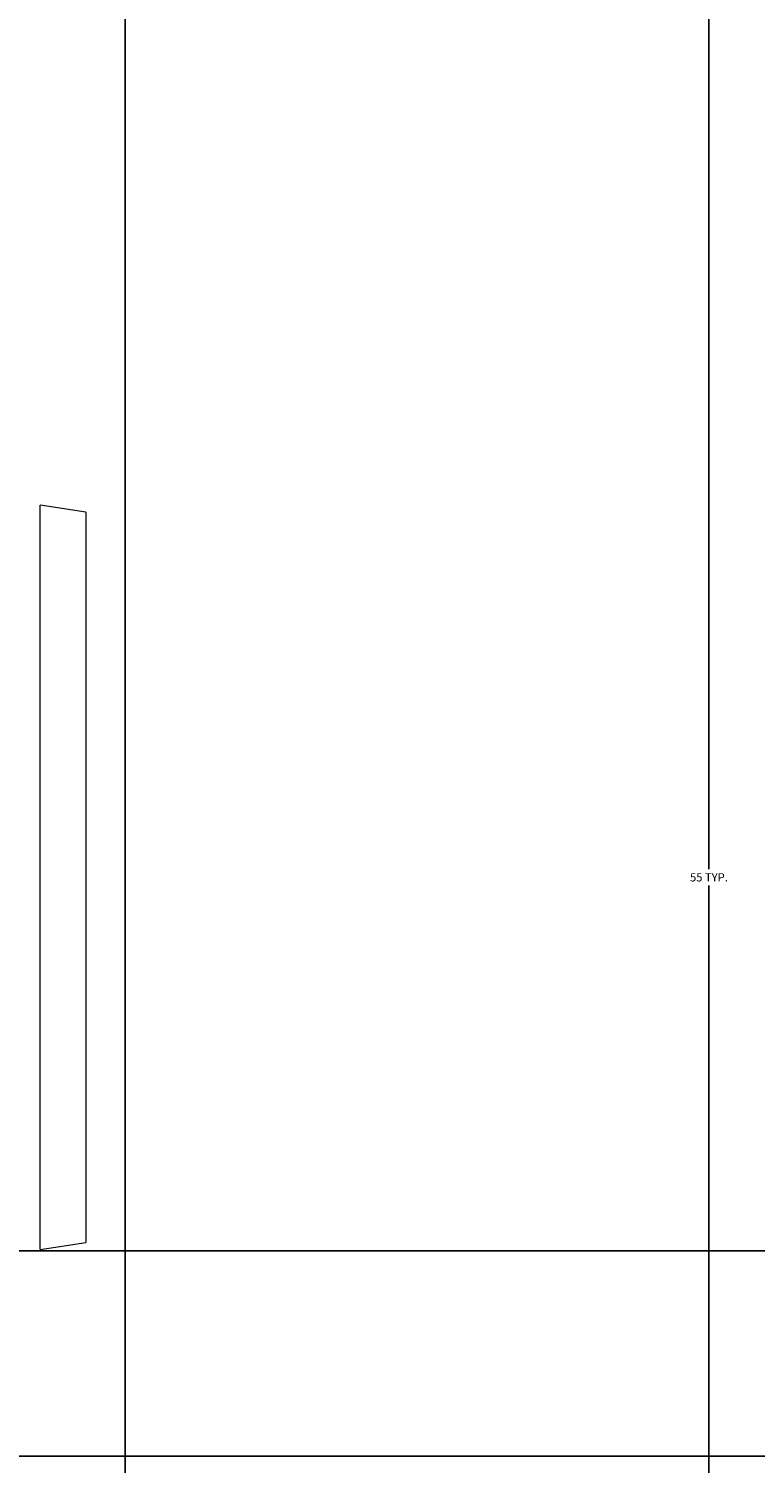
# Model space of a CAD drawing. Units: inches. Extents: x 7359 to 7979, y 33027 to 34263.
# Tile 12 of 32: x 7748 to 7764, y 33386 to 33417. Entities that reach past the tile are written whole.
import ezdxf

# ---------------------------------------------------------------- set-up
doc = ezdxf.new("R2010")
doc.units = ezdxf.units.IN
doc.layers.add('A-ANNO-DIMS', color=2, linetype='Continuous', lineweight=18)
doc.layers.add('A-FURN', color=8, linetype='Continuous', lineweight=18)
doc.styles.get("Standard").update_dxf_attribs({"font": 'arial.ttf'})
doc.dimstyles.get("Standard").update_dxf_attribs({"dimtxt": 0.18, "dimasz": 0.18, "dimexe": 0.18, "dimexo": 0.0625, "dimgap": 0.09, "dimtad": 0, "dimtih": 1, "dimtoh": 1, "dimdec": 4, "dimzin": 0, "dimdsep": 46, "dimtxsty": 'Standard', "dimcen": 0.09, "dimadec": 0, "dimazin": 0, "dimtfac": 1, "dimtdec": 4, "dimtofl": 0, "dimtmove": 0, "dimatfit": 3, "dimfxl": 1, "dimtolj": 1, "dimtzin": 0, "dimarcsym": 0})

# ---------------------------------------------------------------- blocks, each defined once
blk = doc.blocks.new('Dining Set - 36 x 72 in.')
for p, q in [((44.5, -8.15843), (44.5, 8.15338)), ((45.5, 8), (44.5005, 8.15617)), ((45.5, 8), (45.5, -8)), ((44.4997, -8.15631), (45.5, -8))]:
    blk.add_line(p, q)
blk = doc.blocks.new('*D37')
at = {"layer": 'A-ANNO-DIMS', "color": 0, "lineweight": -2, "transparency": 16777216}
for p, q in [((7748.925, 33426.344), (7762.693, 33426.344)), ((7762.513, 33426.164), (7762.513, 33399.025)), ((7762.513, 33371.524), (7762.513, 33398.662)), ((7748.925, 33371.344), (7762.693, 33371.344))]:
    blk.add_line(p, q, dxfattribs=at)
at = {"layer": 'A-ANNO-DIMS', "color": 0, "transparency": 16777216}
for points in [[(7762.483, 33426.164), (7762.543, 33426.164), (7762.513, 33426.344)], [(7762.483, 33371.524), (7762.543, 33371.524), (7762.513, 33371.344)]]:
    blk.add_solid(points, dxfattribs=at)
at = {"layer": 'Defpoints', "color": 0, "transparency": 16777216}
for p in [(7748.863, 33426.344), (7762.513, 33426.344), (7748.863, 33371.344)]:
    blk.add_point(p, dxfattribs=at)
at = {"layer": 'A-ANNO-DIMS', "color": 0, "transparency": 16777216, "insert": (7762.513, 33398.844), "char_height": 0.18, "attachment_point": 5}
blk.add_mtext('\\A1;55 TYP.', dxfattribs=at)
blk = doc.blocks.new('*D74')
at = {"layer": 'A-ANNO-DIMS', "color": 0, "lineweight": -2, "transparency": 16777216}
for p, q in [((7743.727, 33618.1), (7743.727, 33027.177)), ((7787.034, 33618.1), (7787.034, 33027.177)), ((7743.907, 33027.357), (7765, 33027.357)), ((7786.854, 33027.357), (7765.76, 33027.357))]:
    blk.add_line(p, q, dxfattribs=at)
at = {"layer": 'A-ANNO-DIMS', "color": 0, "transparency": 16777216}
for points in [[(7743.907, 33027.387), (7743.907, 33027.327), (7743.727, 33027.357)], [(7786.854, 33027.387), (7786.854, 33027.327), (7787.034, 33027.357)]]:
    blk.add_solid(points, dxfattribs=at)
at = {"layer": 'Defpoints', "color": 0, "transparency": 16777216}
for p in [(7743.727, 33618.162), (7787.034, 33618.162), (7787.034, 33027.357)]:
    blk.add_point(p, dxfattribs=at)
at = {"layer": 'A-ANNO-DIMS', "color": 0, "transparency": 16777216, "insert": (7765.38, 33027.357), "char_height": 0.18, "attachment_point": 5}
blk.add_mtext('\\A1;43.31', dxfattribs=at)
blk = doc.blocks.new('*D85')
at = {"layer": 'A-ANNO-DIMS', "color": 0, "lineweight": -2, "transparency": 16777216}
for p, q in [((7793.064, 33390.662), (7369.542, 33390.662)), ((7369.722, 33390.482), (7369.722, 33388.594)), ((7369.722, 33386.342), (7369.722, 33388.231)), ((7793.064, 33386.162), (7369.542, 33386.162))]:
    blk.add_line(p, q, dxfattribs=at)
at = {"layer": 'A-ANNO-DIMS', "color": 0, "transparency": 16777216}
for points in [[(7369.692, 33390.482), (7369.752, 33390.482), (7369.722, 33390.662)], [(7369.692, 33386.342), (7369.752, 33386.342), (7369.722, 33386.162)]]:
    blk.add_solid(points, dxfattribs=at)
at = {"layer": 'Defpoints', "color": 0, "transparency": 16777216}
for p in [(7793.127, 33390.662), (7369.722, 33386.162), (7793.127, 33386.162)]:
    blk.add_point(p, dxfattribs=at)
at = {"layer": 'A-ANNO-DIMS', "color": 0, "transparency": 16777216, "insert": (7369.722, 33388.412), "char_height": 0.18, "attachment_point": 5}
blk.add_mtext('\\A1;4.5', dxfattribs=at)
blk = doc.blocks.new('*D87')
at = {"layer": 'A-ANNO-DIMS', "color": 0, "lineweight": -2, "transparency": 16777216}
for p, q in [((7743.726578, 33453.099789), (7743.726578, 33027.176807)), ((7749.726578, 33453.099789), (7749.726578, 33027.176807)), ((7743.906578, 33027.356807), (7746.577151, 33027.356807)), ((7749.546578, 33027.356807), (7746.876005, 33027.356807))]:
    blk.add_line(p, q, dxfattribs=at)
at = {"layer": 'A-ANNO-DIMS', "color": 0, "transparency": 16777216}
for points in [[(7743.906578, 33027.386807), (7743.906578, 33027.326807), (7743.726578, 33027.356807)], [(7749.546578, 33027.386807), (7749.546578, 33027.326807), (7749.726578, 33027.356807)]]:
    blk.add_solid(points, dxfattribs=at)
at = {"layer": 'Defpoints', "color": 0, "transparency": 16777216}
for p in [(7743.726578, 33453.162289), (7749.726578, 33453.162289), (7749.726578, 33027.356807)]:
    blk.add_point(p, dxfattribs=at)
at = {"layer": 'A-ANNO-DIMS', "color": 0, "transparency": 16777216, "insert": (7746.726578, 33027.356807), "char_height": 0.18, "attachment_point": 5}
blk.add_mtext('\\A1;6', dxfattribs=at)

msp = doc.modelspace()

# ---------------------------------------------------------------- block references
at = {"layer": 'A-FURN'}
msp.add_blockref('Dining Set - 36 x 72 in.', (7703.363, 33398.8436), dxfattribs=at)

# ---------------------------------------------------------------- dimensions: what is measured, and where the dimension line sits
at = {"layer": 'A-ANNO-DIMS'}
for base, p1, p2, override, picture, middle in [((7787.0342, 33027.3568), (7743.7266, 33618.1623), (7787.0342, 33618.1623), {"dimdec": 2, "dimlfac": 1, "dimrnd": 0, "dimzin": 0, "dimdsep": 46, "dimlunit": 2}, '*D74', (7765.3804, 33027.3568)), ((7749.7266, 33027.3568), (7743.7266, 33453.1623), (7749.7266, 33453.1623), {"dimdec": 0, "dimlfac": 1, "dimrnd": 0, "dimzin": 0, "dimdsep": 46, "dimlunit": 2}, '*D87', (7746.7266, 33027.3568))]:
    dim = msp.add_linear_dim(base=base, p1=p1, p2=p2, dimstyle='Standard', override=override, dxfattribs=at)
    dim.commit()
    dim.dimension.update_dxf_attribs({"geometry": picture, "text_midpoint": middle})
dim = msp.add_linear_dim(base=(7762.513, 33426.3436), p1=(7748.863, 33371.3436), p2=(7748.863, 33426.3436), angle=90, text='<> TYP.', dimstyle='Standard', override={"dimdec": 0, "dimlfac": 1, "dimrnd": 0, "dimzin": 0, "dimdsep": 46, "dimlunit": 2}, dxfattribs=at)
dim.commit()
dim.dimension.update_dxf_attribs({"geometry": '*D37', "text_midpoint": (7762.513, 33398.8436)})
dim = msp.add_linear_dim(base=(7369.7217, 33386.1623), p1=(7793.1266, 33390.6623), p2=(7793.1266, 33386.1623), angle=90, dimstyle='Standard', override={"dimdec": 1, "dimlfac": 1, "dimrnd": 0, "dimzin": 0, "dimdsep": 46, "dimlunit": 2}, dxfattribs=at)
dim.commit()
dim.dimension.update_dxf_attribs({"geometry": '*D85', "text_midpoint": (7369.7217, 33388.4123)})

doc.saveas('drawing.dxf')
